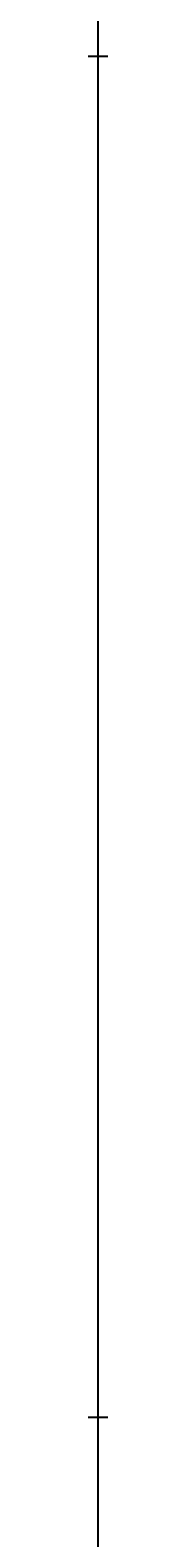
# Model space of a CAD drawing. Units: inches. Extents: x 35362 to 73946, y 43607 to 67532.
# Tile 40 of 134: x 48373 to 48373, y 46091 to 46564. Entities that reach past the tile are written whole.
import ezdxf

# ---------------------------------------------------------------- set-up
doc = ezdxf.new("R2010")
doc.units = ezdxf.units.IN
doc.header["$MEASUREMENT"] = 0
doc.layers.add('A-ANNO-DIMS', color=2, linetype='Continuous', lineweight=18)
doc.styles.get("Standard").update_dxf_attribs({"font": 'arial.ttf'})
doc.dimstyles.get("Standard").update_dxf_attribs({"dimtxt": 0.18, "dimasz": 0.18, "dimexe": 0.18, "dimexo": 0.0625, "dimgap": 0.09, "dimtad": 0, "dimtih": 1, "dimtoh": 1, "dimdec": 4, "dimzin": 0, "dimdsep": 46, "dimtxsty": 'Standard', "dimcen": 0.09, "dimadec": 0, "dimazin": 0, "dimtfac": 1, "dimtdec": 4, "dimtofl": 0, "dimtmove": 0, "dimatfit": 3, "dimfxl": 1, "dimtolj": 1, "dimtzin": 0, "dimarcsym": 0})

# ---------------------------------------------------------------- blocks, each defined once
blk = doc.blocks.new('*D5')
at = {"layer": 'A-ANNO-DIMS', "color": 0, "lineweight": -2, "transparency": 16777216}
for p, q in [((37121.95, 46919.32), (37121.95, 43606.68)), ((69871.5, 45449.83), (69871.5, 43606.68)), ((37122.13, 43606.86), (53496.29, 43606.86)), ((69871.32, 43606.86), (53497.15, 43606.86))]:
    blk.add_line(p, q, dxfattribs=at)
at = {"layer": 'A-ANNO-DIMS', "color": 0, "transparency": 16777216}
for points in [[(37122.13, 43606.89), (37122.13, 43606.83), (37121.95, 43606.86)], [(69871.32, 43606.89), (69871.32, 43606.83), (69871.5, 43606.86)]]:
    blk.add_solid(points, dxfattribs=at)
at = {"layer": 'Defpoints', "color": 0, "transparency": 16777216}
for p in [(37121.95, 46919.38), (69871.5, 45449.89), (69871.5, 43606.86)]:
    blk.add_point(p, dxfattribs=at)
at = {"layer": 'A-ANNO-DIMS', "color": 0, "transparency": 16777216, "insert": (53496.72, 43606.86), "char_height": 0.18, "attachment_point": 5}
blk.add_mtext('\\A1;32750', dxfattribs=at)
blk = doc.blocks.new('*D11')
at = {"layer": 'A-ANNO-DIMS', "color": 0, "lineweight": -2, "transparency": 16777216}
for p, q in [((47978.66, 56028.77), (47978.66, 43606.68)), ((53109.76, 56028.77), (53109.76, 43606.68)), ((47978.84, 43606.86), (50543.87, 43606.86)), ((53109.58, 43606.86), (50544.55, 43606.86))]:
    blk.add_line(p, q, dxfattribs=at)
at = {"layer": 'A-ANNO-DIMS', "color": 0, "transparency": 16777216}
for points in [[(47978.84, 43606.89), (47978.84, 43606.83), (47978.66, 43606.86)], [(53109.58, 43606.89), (53109.58, 43606.83), (53109.76, 43606.86)]]:
    blk.add_solid(points, dxfattribs=at)
at = {"layer": 'Defpoints', "color": 0, "transparency": 16777216}
for p in [(47978.66, 56028.84), (53109.76, 56028.84), (53109.76, 43606.86)]:
    blk.add_point(p, dxfattribs=at)
at = {"layer": 'A-ANNO-DIMS', "color": 0, "transparency": 16777216, "insert": (50544.21, 43606.86), "char_height": 0.18, "attachment_point": 5}
blk.add_mtext('\\A1;5131', dxfattribs=at)
blk = doc.blocks.new('*D13')
at = {"layer": 'A-ANNO-DIMS', "color": 0, "lineweight": -2, "transparency": 16777216}
for p, q in [((48373.49, 51694.02), (48373.49, 43606.68)), ((51029.04, 51694.02), (51029.04, 43606.68)), ((48373.67, 43606.86), (49700.8, 43606.86)), ((51028.86, 43606.86), (49701.73, 43606.86))]:
    blk.add_line(p, q, dxfattribs=at)
at = {"layer": 'A-ANNO-DIMS', "color": 0, "transparency": 16777216}
for points in [[(48373.67, 43606.89), (48373.67, 43606.83), (48373.49, 43606.86)], [(51028.86, 43606.89), (51028.86, 43606.83), (51029.04, 43606.86)]]:
    blk.add_solid(points, dxfattribs=at)
at = {"layer": 'Defpoints', "color": 0, "transparency": 16777216}
for p in [(48373.49, 51694.09), (51029.04, 51694.09), (51029.04, 43606.86)]:
    blk.add_point(p, dxfattribs=at)
at = {"layer": 'A-ANNO-DIMS', "color": 0, "transparency": 16777216, "insert": (49701.27, 43606.86), "char_height": 0.18, "attachment_point": 5}
blk.add_mtext('\\A1;2655.6', dxfattribs=at)
blk = doc.blocks.new('*D67')
at = {"layer": 'A-ANNO-DIMS', "color": 0, "lineweight": -2, "transparency": 16777216}
for p, q in [((56873.54, 53351.53), (35361.77, 53351.53)), ((35361.95, 53351.35), (35361.95, 49400.89)), ((35361.95, 45450.07), (35361.95, 49400.53)), ((53793.58, 45449.89), (35361.77, 45449.89))]:
    blk.add_line(p, q, dxfattribs=at)
at = {"layer": 'A-ANNO-DIMS', "color": 0, "transparency": 16777216}
for points in [[(35361.92, 53351.35), (35361.98, 53351.35), (35361.95, 53351.53)], [(35361.92, 45450.07), (35361.98, 45450.07), (35361.95, 45449.89)]]:
    blk.add_solid(points, dxfattribs=at)
at = {"layer": 'Defpoints', "color": 0, "transparency": 16777216}
for p in [(35361.95, 53351.53), (56873.6, 53351.53), (53793.64, 45449.89)]:
    blk.add_point(p, dxfattribs=at)
at = {"layer": 'A-ANNO-DIMS', "color": 0, "transparency": 16777216, "insert": (35361.95, 49400.71), "char_height": 0.18, "attachment_point": 5}
blk.add_mtext('\\A1;7901.6', dxfattribs=at)
blk = doc.blocks.new('*D76')
at = {"layer": 'A-ANNO-DIMS', "color": 0, "lineweight": -2, "transparency": 16777216}
for p, q in [((54052.84, 46555.29), (35361.77, 46555.29)), ((35361.95, 46555.11), (35361.95, 46342.27)), ((35361.95, 46129.06), (35361.95, 46341.9)), ((53793.58, 46128.88), (35361.77, 46128.88))]:
    blk.add_line(p, q, dxfattribs=at)
at = {"layer": 'A-ANNO-DIMS', "color": 0, "transparency": 16777216}
for points in [[(35361.92, 46555.11), (35361.98, 46555.11), (35361.95, 46555.29)], [(35361.92, 46129.06), (35361.98, 46129.06), (35361.95, 46128.88)]]:
    blk.add_solid(points, dxfattribs=at)
at = {"layer": 'Defpoints', "color": 0, "transparency": 16777216}
for p in [(35361.95, 46555.29), (54052.9, 46555.29), (53793.64, 46128.88)]:
    blk.add_point(p, dxfattribs=at)
at = {"layer": 'A-ANNO-DIMS', "color": 0, "transparency": 16777216, "insert": (35361.95, 46342.09), "char_height": 0.18, "attachment_point": 5}
blk.add_mtext('\\A1;426.4', dxfattribs=at)
blk = doc.blocks.new('*D90')
at = {"layer": 'A-ANNO-DIMS', "color": 0, "lineweight": -2, "transparency": 16777216}
for p, q in [((53707.72, 47291.29), (35361.77, 47291.29)), ((35361.95, 47291.11), (35361.95, 46710.26)), ((35361.95, 46129.06), (35361.95, 46709.9)), ((53793.58, 46128.88), (35361.77, 46128.88))]:
    blk.add_line(p, q, dxfattribs=at)
at = {"layer": 'A-ANNO-DIMS', "color": 0, "transparency": 16777216}
for points in [[(35361.92, 47291.11), (35361.98, 47291.11), (35361.95, 47291.29)], [(35361.92, 46129.06), (35361.98, 46129.06), (35361.95, 46128.88)]]:
    blk.add_solid(points, dxfattribs=at)
at = {"layer": 'Defpoints', "color": 0, "transparency": 16777216}
for p in [(53707.78, 47291.29), (35361.95, 46128.88), (53793.64, 46128.88)]:
    blk.add_point(p, dxfattribs=at)
at = {"layer": 'A-ANNO-DIMS', "color": 0, "transparency": 16777216, "insert": (35361.95, 46710.08), "char_height": 0.18, "attachment_point": 5}
blk.add_mtext('\\A1;1162.4', dxfattribs=at)

msp = doc.modelspace()

# ---------------------------------------------------------------- dimensions: what is measured, and where the dimension line sits
at = {"layer": 'A-ANNO-DIMS'}
for base, p1, p2, override, picture, middle in [((53109.76, 43606.859), (47978.665, 56028.836), (53109.76, 56028.836), {"dimdec": 0, "dimlfac": 1, "dimrnd": 0, "dimzin": 0, "dimdsep": 46, "dimlunit": 2}, '*D11', (50544.212, 43606.859)), ((51029.043, 43606.859), (48373.492, 51694.087), (51029.043, 51694.087), {"dimdec": 1, "dimlfac": 1, "dimrnd": 0, "dimzin": 0, "dimdsep": 46, "dimlunit": 2}, '*D13', (49701.267, 43606.859)), ((69871.496, 43606.859), (37121.949, 46919.381), (69871.496, 45449.894), {"dimdec": 0, "dimlfac": 1, "dimrnd": 0, "dimzin": 0, "dimdsep": 46, "dimlunit": 2}, '*D5', (53496.723, 43606.859))]:
    dim = msp.add_linear_dim(base=base, p1=p1, p2=p2, dimstyle='Standard', override=override, dxfattribs=at)
    dim.commit()
    dim.dimension.update_dxf_attribs({"geometry": picture, "text_midpoint": middle})
for base, p1, p2, picture, middle in [((35361.949, 53351.529), (53793.638, 45449.894), (56873.602, 53351.529), '*D67', (35361.949, 49400.712)), ((35361.949, 46128.878), (53707.781, 47291.285), (53793.638, 46128.878), '*D90', (35361.949, 46710.081)), ((35361.949, 46555.293), (53793.638, 46128.878), (54052.899, 46555.293), '*D76', (35361.949, 46342.086))]:
    dim = msp.add_linear_dim(base=base, p1=p1, p2=p2, angle=90, dimstyle='Standard', override={"dimdec": 1, "dimlfac": 1, "dimrnd": 0, "dimzin": 0, "dimdsep": 46, "dimlunit": 2}, dxfattribs=at)
    dim.commit()
    dim.dimension.update_dxf_attribs({"geometry": picture, "text_midpoint": middle})

doc.saveas('drawing.dxf')
